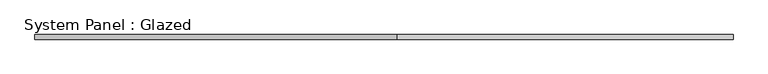
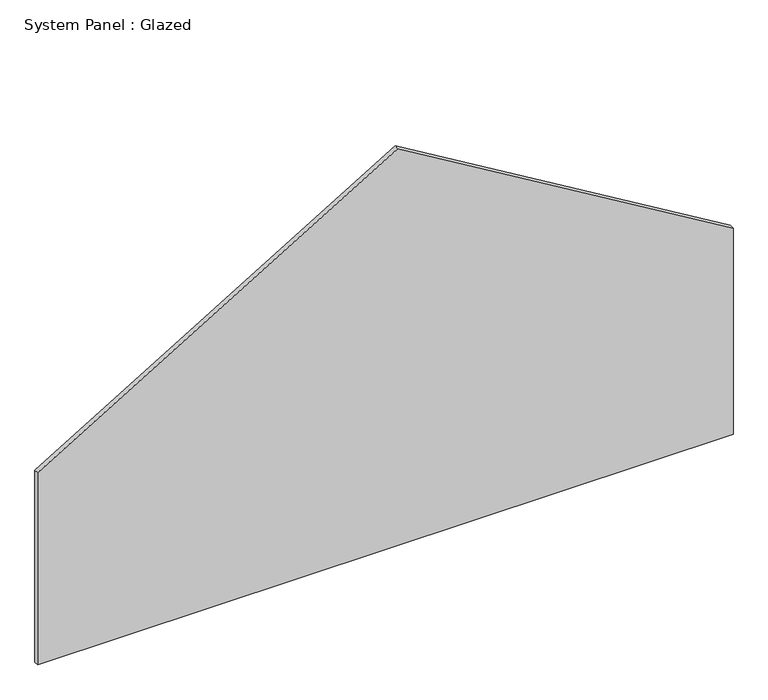
"""IFC4 building model written with IfcOpenShell, lengths in millimetres: plate geometry, System Panel : Glazed."""

from ifc_helpers import new_model, si_unit, frame, origin, place, context, project, spatial, polyline, outline, extrude, source, transform, mapped, element, save


def system_panel_glazed_24e5f3e2(model_context):
    return source(origin(), model_context, "Body", "SweptSolid", [
        extrude(outline(polyline([(0.0, -1930.4), (0.0, 1930.4), (1211.2644616, 1930.4), (2329.1956864, 69.85), (1127.3242332, -1930.4), (0.0, -1930.4)])), frame((0.0, 19.05, 0.0), z_axis=(0.0, 1.0, 0.0), x_axis=(0.0, 0.0, 1.0)), (0.0, 0.0, 1.0), 25.4),
    ])


if __name__ == "__main__":
    model = new_model("IFC4")
    model_context = context("Model", 3, world=origin())
    ifc_project = project(units=[si_unit("LENGTHUNIT", "METRE", prefix="MILLI")], contexts=[model_context])
    site = spatial("IfcSite", under=ifc_project)
    building = spatial("IfcBuilding", under=site)
    placement = place(None, origin())
    system_panel_glazed_shape = system_panel_glazed_24e5f3e2(model_context)
    element("IfcPlate", 1, ObjectType="System Panel : Glazed", at=placement, inside=building, context=model_context, shape_type="MappedRepresentation", body=[
        mapped(system_panel_glazed_shape, transform((0.0, 0.0, 0.0), x_axis=(1.0, 0.0, 0.0), y_axis=(0.0, 1.0, 0.0), z_axis=(0.0, 0.0, 1.0))),
    ])
    save(model, "model.ifc")

# Revit data of these elements
# Type "System Panel : Glazed"
#   Construction Type Id = "GSP4R"
#   Analytic Construction = "1/8 in Pilkington single glazing"
#   Visual Light Transmittance = 0.9
#   Solar Heat Gain Coefficient = 0.86
#   Heat Transfer Coefficient (U) = 1.18115 BTU/(h·ft²·°F)
#   Define Thermal Properties by = 1
# Element 1 (IfcPlate, "System Panel : Glazed")
#   Materials on its faces: "Glass"
# Materials
#   "Glass": class "Glass", colour RGB 0 128 192, transparency 0.75, Description = "Soda Lime Glass", Cost = 0
